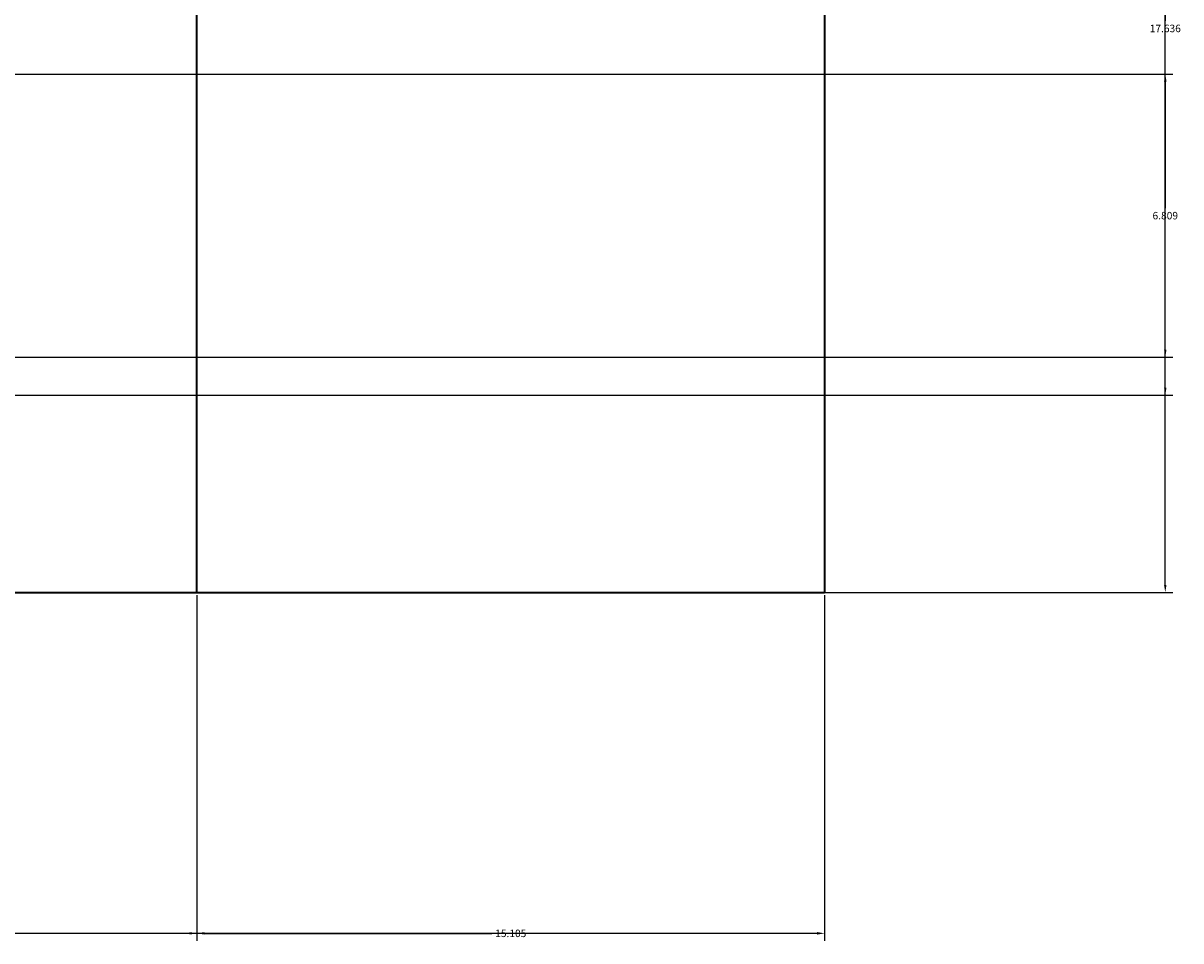
# Model space of a CAD drawing. Units: inches. Extents: x 27 to 200, y -50 to 102.
# Tile 14 of 26: x 172 to 200, y -25 to -3. Entities that reach past the tile are written whole.
import ezdxf

# ---------------------------------------------------------------- set-up
doc = ezdxf.new("R2010")
doc.units = ezdxf.units.IN
doc.header["$MEASUREMENT"] = 0
doc.layers.add('A-ANNO-DIMS', color=2, linetype='Continuous', lineweight=18)
doc.layers.add('A-ELEV', color=7, linetype='Continuous', lineweight=35)
doc.styles.get("Standard").update_dxf_attribs({"font": 'arial.ttf'})
doc.dimstyles.get("Standard").update_dxf_attribs({"dimtxt": 0.18, "dimasz": 0.18, "dimexe": 0.18, "dimexo": 0.0625, "dimgap": 0.09, "dimtad": 0, "dimtih": 1, "dimtoh": 1, "dimdec": 4, "dimzin": 0, "dimdsep": 46, "dimtxsty": 'Standard', "dimcen": 0.09, "dimadec": 0, "dimazin": 0, "dimtfac": 1, "dimtdec": 4, "dimtofl": 0, "dimtmove": 0, "dimatfit": 3, "dimfxl": 1, "dimtolj": 1, "dimtzin": 0, "dimarcsym": 0})

# ---------------------------------------------------------------- blocks, each defined once
blk = doc.blocks.new('*D23')
at = {"layer": 'A-ANNO-DIMS', "color": 0, "lineweight": -2, "transparency": 16777216}
for p, q in [((35.417, -16.832), (35.417, -25.149)), ((191.417, -16.832), (191.417, -25.149)), ((35.597, -24.969), (113.137, -24.969)), ((191.237, -24.969), (113.697, -24.969))]:
    blk.add_line(p, q, dxfattribs=at)
at = {"layer": 'A-ANNO-DIMS', "color": 0, "transparency": 16777216}
for points in [[(35.597, -24.939), (35.597, -24.999), (35.417, -24.969)], [(191.237, -24.939), (191.237, -24.999), (191.417, -24.969)]]:
    blk.add_solid(points, dxfattribs=at)
at = {"layer": 'Defpoints', "color": 0, "transparency": 16777216}
for p in [(35.417, -16.769), (191.417, -16.769), (191.417, -24.969)]:
    blk.add_point(p, dxfattribs=at)
at = {"layer": 'A-ANNO-DIMS', "color": 0, "transparency": 16777216, "insert": (113.417, -24.969), "char_height": 0.18, "attachment_point": 5}
blk.add_mtext('\\A1;156', dxfattribs=at)
blk = doc.blocks.new('*D25')
at = {"layer": 'A-ANNO-DIMS', "color": 0, "lineweight": -2, "transparency": 16777216}
for p, q in [((191.473, 16.002), (199.797, 16.002)), ((199.617, 15.822), (199.617, -0.202)), ((199.617, -16.589), (199.617, -0.566)), ((191.479, -16.769), (199.797, -16.769))]:
    blk.add_line(p, q, dxfattribs=at)
at = {"layer": 'A-ANNO-DIMS', "color": 0, "transparency": 16777216}
for points in [[(199.587, 15.822), (199.647, 15.822), (199.617, 16.002)], [(199.587, -16.589), (199.647, -16.589), (199.617, -16.769)]]:
    blk.add_solid(points, dxfattribs=at)
at = {"layer": 'Defpoints', "color": 0, "transparency": 16777216}
for p in [(191.41, 16.002), (199.617, 16.002), (191.417, -16.769)]:
    blk.add_point(p, dxfattribs=at)
at = {"layer": 'A-ANNO-DIMS', "color": 0, "transparency": 16777216, "insert": (199.617, -0.384), "char_height": 0.18, "attachment_point": 5}
blk.add_mtext('\\A1;32.77', dxfattribs=at)
blk = doc.blocks.new('*D39')
at = {"layer": 'A-ANNO-DIMS', "color": 0, "lineweight": -2, "transparency": 16777216}
for p, q in [((167.312, -16.832), (167.312, -25.149)), ((176.312, -16.832), (176.312, -25.149)), ((167.492, -24.969), (171.663, -24.969)), ((176.132, -24.969), (171.961, -24.969))]:
    blk.add_line(p, q, dxfattribs=at)
at = {"layer": 'A-ANNO-DIMS', "color": 0, "transparency": 16777216}
for points in [[(167.492, -24.939), (167.492, -24.999), (167.312, -24.969)], [(176.132, -24.939), (176.132, -24.999), (176.312, -24.969)]]:
    blk.add_solid(points, dxfattribs=at)
at = {"layer": 'Defpoints', "color": 0, "transparency": 16777216}
for p in [(167.312, -16.769), (176.312, -16.769), (176.312, -24.969)]:
    blk.add_point(p, dxfattribs=at)
at = {"layer": 'A-ANNO-DIMS', "color": 0, "transparency": 16777216, "insert": (171.812, -24.969), "char_height": 0.18, "attachment_point": 5}
blk.add_mtext('\\A1;9', dxfattribs=at)
blk = doc.blocks.new('*D40')
at = {"layer": 'A-ANNO-DIMS', "color": 0, "lineweight": -2, "transparency": 16777216}
for p, q in [((176.312, -16.832), (176.312, -25.149)), ((191.417, -16.832), (191.417, -25.149)), ((176.492, -24.969), (183.409, -24.969)), ((191.237, -24.969), (184.32, -24.969))]:
    blk.add_line(p, q, dxfattribs=at)
at = {"layer": 'A-ANNO-DIMS', "color": 0, "transparency": 16777216}
for points in [[(176.492, -24.939), (176.492, -24.999), (176.312, -24.969)], [(191.237, -24.939), (191.237, -24.999), (191.417, -24.969)]]:
    blk.add_solid(points, dxfattribs=at)
at = {"layer": 'Defpoints', "color": 0, "transparency": 16777216}
for p in [(176.312, -16.769), (191.417, -16.769), (191.417, -24.969)]:
    blk.add_point(p, dxfattribs=at)
at = {"layer": 'A-ANNO-DIMS', "color": 0, "transparency": 16777216, "insert": (183.864, -24.969), "char_height": 0.18, "attachment_point": 5}
blk.add_mtext('\\A1;15.105', dxfattribs=at)
blk = doc.blocks.new('*D48')
at = {"layer": 'A-ANNO-DIMS', "color": 0, "lineweight": -2, "transparency": 16777216}
for p, q in [((84.479, 44.926), (199.797, 44.926)), ((199.617, 44.746), (199.617, 14.26)), ((199.617, -16.589), (199.617, 13.897)), ((84.479, -16.769), (199.797, -16.769))]:
    blk.add_line(p, q, dxfattribs=at)
at = {"layer": 'A-ANNO-DIMS', "color": 0, "transparency": 16777216}
for points in [[(199.587, 44.746), (199.647, 44.746), (199.617, 44.926)], [(199.587, -16.589), (199.647, -16.589), (199.617, -16.769)]]:
    blk.add_solid(points, dxfattribs=at)
at = {"layer": 'Defpoints', "color": 0, "transparency": 16777216}
for p in [(84.417, 44.926), (199.617, 44.926), (84.417, -16.769)]:
    blk.add_point(p, dxfattribs=at)
at = {"layer": 'A-ANNO-DIMS', "color": 0, "transparency": 16777216, "insert": (199.617, 14.079), "char_height": 0.18, "attachment_point": 5}
blk.add_mtext('\\A1;61.7', dxfattribs=at)
blk = doc.blocks.new('*D62')
at = {"layer": 'A-ANNO-DIMS', "color": 0, "lineweight": -2, "transparency": 16777216}
for p, q in [((140.41, -4.3), (199.797, -4.3)), ((199.617, -4.48), (199.617, -7.522)), ((199.617, -10.928), (199.617, -7.886)), ((140.41, -11.108), (199.797, -11.108))]:
    blk.add_line(p, q, dxfattribs=at)
at = {"layer": 'A-ANNO-DIMS', "color": 0, "transparency": 16777216}
for points in [[(199.587, -4.48), (199.647, -4.48), (199.617, -4.3)], [(199.587, -10.928), (199.647, -10.928), (199.617, -11.108)]]:
    blk.add_solid(points, dxfattribs=at)
at = {"layer": 'Defpoints', "color": 0, "transparency": 16777216}
for p in [(140.347, -4.3), (199.617, -4.3), (140.347, -11.108)]:
    blk.add_point(p, dxfattribs=at)
at = {"layer": 'A-ANNO-DIMS', "color": 0, "transparency": 16777216, "insert": (199.617, -7.704), "char_height": 0.18, "attachment_point": 5}
blk.add_mtext('\\A1;6.809', dxfattribs=at)
blk = doc.blocks.new('*D67')
at = {"layer": 'A-ANNO-DIMS', "color": 0, "lineweight": -2, "transparency": 16777216}
for p, q in [((165.546, 5.617), (199.797, 5.617)), ((199.617, 5.437), (199.617, -3.019)), ((199.617, -11.839), (199.617, -3.383)), ((165.546, -12.019), (199.797, -12.019))]:
    blk.add_line(p, q, dxfattribs=at)
at = {"layer": 'A-ANNO-DIMS', "color": 0, "transparency": 16777216}
for points in [[(199.587, 5.437), (199.647, 5.437), (199.617, 5.617)], [(199.587, -11.839), (199.647, -11.839), (199.617, -12.019)]]:
    blk.add_solid(points, dxfattribs=at)
at = {"layer": 'Defpoints', "color": 0, "transparency": 16777216}
for p in [(165.484, 5.617), (199.617, 5.617), (165.484, -12.019)]:
    blk.add_point(p, dxfattribs=at)
at = {"layer": 'A-ANNO-DIMS', "color": 0, "transparency": 16777216, "insert": (199.617, -3.201), "char_height": 0.18, "attachment_point": 5}
blk.add_mtext('\\A1;17.636', dxfattribs=at)

msp = doc.modelspace()

# ---------------------------------------------------------------- linework, layer by layer
at = {"layer": 'A-ELEV'}
for p, q in [((191.4169, 93.9264), (191.4169, -16.7693)), ((176.3118, -16.7693), (176.3118, 16.0358)), ((35.4169, -16.7693), (191.4169, -16.7693))]:
    msp.add_line(p, q, dxfattribs=at)

# ---------------------------------------------------------------- dimensions: what is measured, and where the dimension line sits
at = {"layer": 'A-ANNO-DIMS'}
for base, p1, p2, override, picture, middle in [((199.6169, 44.9264), (84.4169, -16.7693), (84.4169, 44.9264), {"dimdec": 1, "dimlfac": 1, "dimrnd": 0, "dimzin": 0, "dimdsep": 46, "dimlunit": 2}, '*D48', (199.6169, 14.0786)), ((199.6169, 16.002), (191.4169, -16.7693), (191.4102, 16.002), {"dimdec": 2, "dimlfac": 1, "dimrnd": 0, "dimzin": 0, "dimdsep": 46, "dimlunit": 2}, '*D25', (199.6169, -0.3836)), ((199.6169, 5.6167), (165.4839, -12.0191), (165.4839, 5.6167), {"dimdec": 3, "dimlfac": 1, "dimrnd": 0, "dimzin": 0, "dimdsep": 46, "dimlunit": 2}, '*D67', (199.6169, -3.2012)), ((199.6169, -4.2997), (140.3471, -11.1085), (140.3471, -4.2997), {"dimdec": 3, "dimlfac": 1, "dimrnd": 0, "dimzin": 0, "dimdsep": 46, "dimlunit": 2}, '*D62', (199.6169, -7.7041))]:
    dim = msp.add_linear_dim(base=base, p1=p1, p2=p2, angle=90, dimstyle='Standard', override=override, dxfattribs=at)
    dim.commit()
    dim.dimension.update_dxf_attribs({"geometry": picture, "text_midpoint": middle})
for base, p1, p2, override, picture, middle in [((191.4169, -24.9693), (35.4169, -16.7693), (191.4169, -16.7693), {"dimdec": 0, "dimlfac": 1, "dimrnd": 0, "dimzin": 0, "dimdsep": 46, "dimlunit": 2}, '*D23', (113.4169, -24.9693)), ((176.3118, -24.9693), (167.3118, -16.7693), (176.3118, -16.7693), {"dimdec": 0, "dimlfac": 1, "dimrnd": 0, "dimzin": 0, "dimdsep": 46, "dimlunit": 2}, '*D39', (171.8118, -24.9693)), ((191.4169, -24.9693), (176.3118, -16.7693), (191.4169, -16.7693), {"dimdec": 3, "dimlfac": 1, "dimrnd": 0, "dimzin": 0, "dimdsep": 46, "dimlunit": 2}, '*D40', (183.8644, -24.9693))]:
    dim = msp.add_linear_dim(base=base, p1=p1, p2=p2, dimstyle='Standard', override=override, dxfattribs=at)
    dim.commit()
    dim.dimension.update_dxf_attribs({"geometry": picture, "text_midpoint": middle})

doc.saveas('drawing.dxf')
